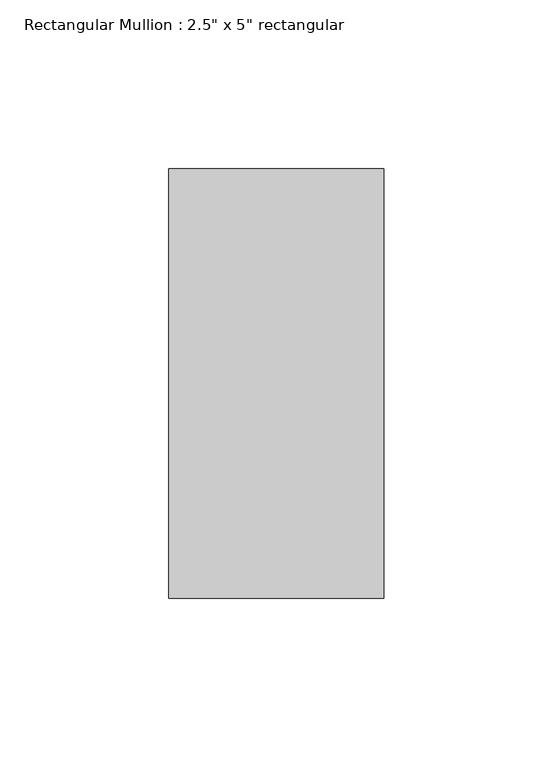
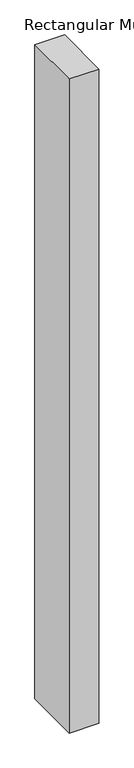
"""IFC4 building model written with IfcOpenShell, lengths in millimetres: member geometry."""

from ifc_helpers import new_model, si_unit, frame, origin, place, context, project, spatial, polyline, outline, extrude, source, transform, mapped, element, save


def member_1fe8360d(model_context):
    return source(origin(), model_context, "Body", "SweptSolid", [
        extrude(outline(polyline([(31.75, 63.5), (31.75, -63.5), (-31.75, -63.5), (-31.75, 63.5), (31.75, 63.5)])), frame((0.0, 0.0, -1477.1971055), z_axis=(0.0, 0.0, 1.0), x_axis=(1.0, 0.0, 0.0)), (0.0, 0.0, 1.0), 1477.1971055),
    ])


if __name__ == "__main__":
    model = new_model("IFC4")
    model_context = context("Model", 3, world=origin())
    ifc_project = project(units=[si_unit("LENGTHUNIT", "METRE", prefix="MILLI")], contexts=[model_context])
    site = spatial("IfcSite", under=ifc_project)
    building = spatial("IfcBuilding", under=site)
    placement = place(None, origin())
    member_shape = member_1fe8360d(model_context)
    element("IfcMember", 1, ObjectType="Rectangular Mullion : 2.5\" x 5\" rectangular", at=placement, inside=building, context=model_context, shape_type="MappedRepresentation", body=[
        mapped(member_shape, transform((0.0, 0.0, 0.0), x_axis=(1.0, 0.0, 0.0), y_axis=(0.0, 1.0, 0.0), z_axis=(0.0, 0.0, 1.0))),
    ])
    save(model, "model.ifc")

# Revit data of these elements
# Type "Rectangular Mullion : 2.5\" x 5\" rectangular"
#   built-in parameter 1007304 = 0.416667 (stored number, unit not read)
#   built-in parameter 1007301 = 0.104167 (stored number, unit not read)
#   built-in parameter 1007300 = 0.104167 (stored number, unit not read)
# Element 1 (IfcMember, "Rectangular Mullion : 2.5\" x 5\" rectangular")
#   Materials on its faces: "Aluminum"
# Materials
#   "Aluminum": class "Metal", colour RGB 247 247 247, transparency 0, Description = "Aluminum 6061", Cost = 0
